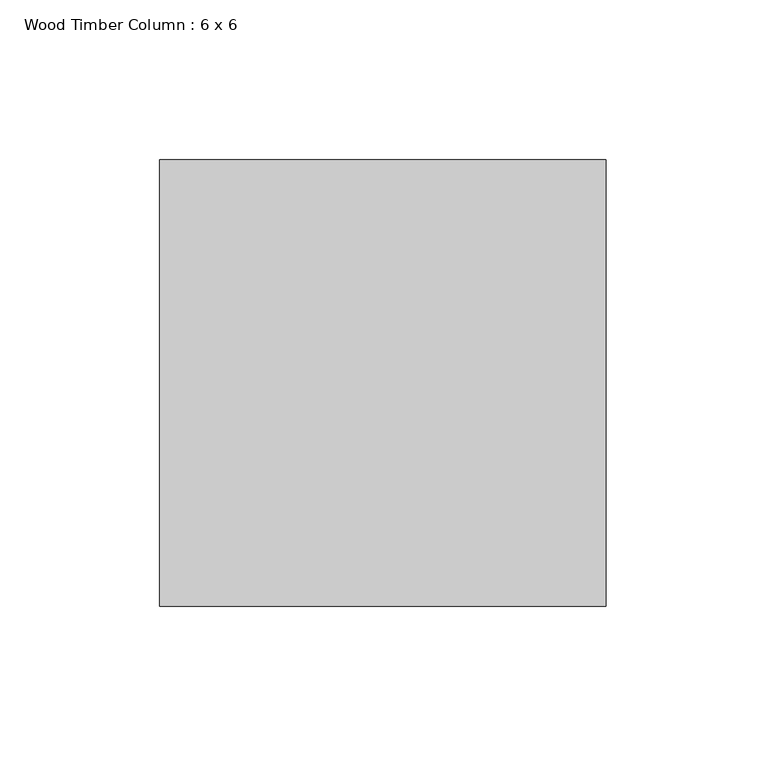
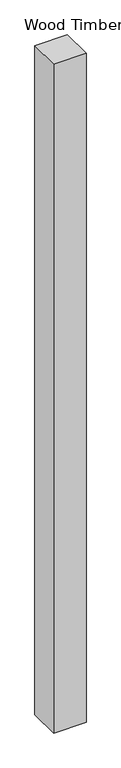
"""IFC4 building model written with IfcOpenShell, lengths in millimetres: column geometry, Wood Timber Column : 6 x 6."""

from ifc_helpers import new_model, si_unit, frame, origin, place, context, project, spatial, polyline, outline, extrude, source, transform, mapped, element, save


def wood_timber_column_6_x_6_20b6f3f8(model_context):
    return source(origin(), model_context, "Body", "SweptSolid", [
        extrude(outline(polyline([(69.85, -69.85), (-69.85, -69.85), (-69.85, 69.85), (69.85, 69.85), (69.85, -69.85)])), frame((0.0, 0.0, 18288.0), z_axis=(0.0, 0.0, 1.0), x_axis=(1.0, 0.0, 0.0)), (0.0, 0.0, 1.0), 3048.0),
    ])


if __name__ == "__main__":
    model = new_model("IFC4")
    model_context = context("Model", 3, world=origin())
    ifc_project = project(units=[si_unit("LENGTHUNIT", "METRE", prefix="MILLI")], contexts=[model_context])
    site = spatial("IfcSite", under=ifc_project)
    building = spatial("IfcBuilding", under=site)
    placement = place(None, origin())
    wood_timber_column_6_x_6_shape = wood_timber_column_6_x_6_20b6f3f8(model_context)
    element("IfcColumn", 1, ObjectType="Wood Timber Column : 6 x 6", at=placement, inside=building, context=model_context, shape_type="MappedRepresentation", body=[
        mapped(wood_timber_column_6_x_6_shape, transform((0.0, 0.0, 0.0), x_axis=(1.0, 0.0, 0.0), y_axis=(0.0, 1.0, 0.0), z_axis=(0.0, 0.0, 1.0))),
    ])
    save(model, "model.ifc")

# Revit data of these elements
# Type "Wood Timber Column : 6 x 6"
#   Assembly Code = "B1010200"
#   Depth = 0' - 5 1/2"
#   Width = 0' - 5 1/2"
#   Material = Softwood, Lumber
# Element 1 (IfcColumn, "Wood Timber Column : 6 x 6")
#   Materials on its faces: "Softwood, Lumber"
# Materials
#   "Softwood, Lumber": class "Wood", colour RGB 223 192 134, transparency 0, Description = "Pinus Echinata", Cost = 0
